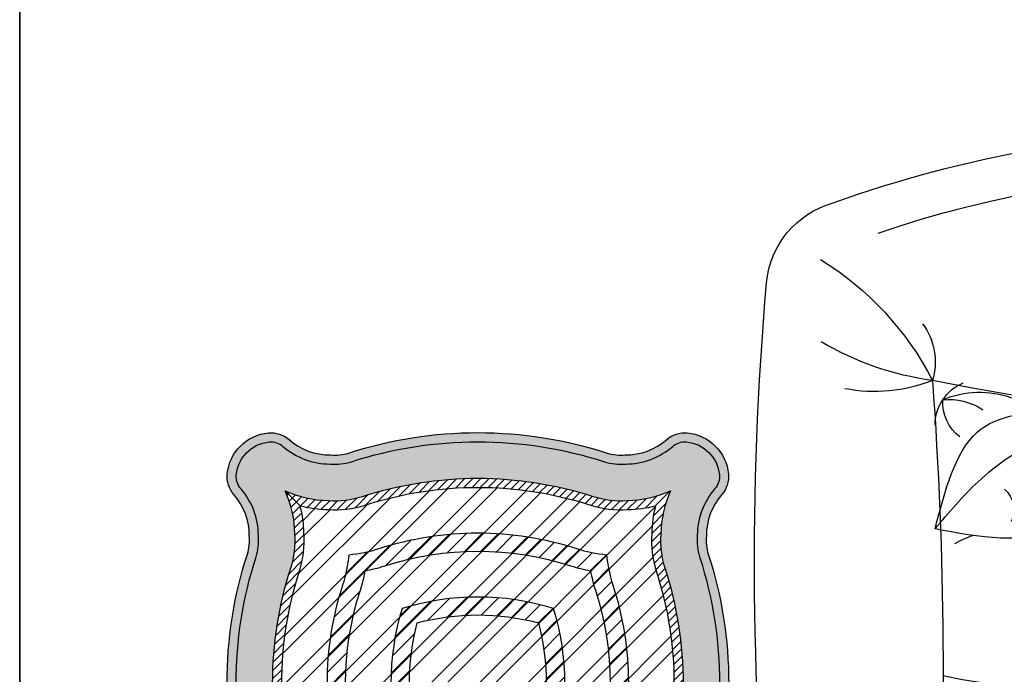
# Model space of a CAD drawing. Units: inches. Extents: x 844 to 2234, y 346 to 1084.
# Tile 63 of 93: x 1843.1 to 1860.31, y 724.36 to 735.81. Entities that reach past the tile are written whole.
import ezdxf

# ---------------------------------------------------------------- set-up
doc = ezdxf.new("R2010")
doc.units = ezdxf.units.IN
doc.header["$MEASUREMENT"] = 0
doc.layers.add('A-WALL', color=7, linetype='Continuous', lineweight=35)
doc.layers.add('furniture', color=8, linetype='Continuous', lineweight=18)
for name, color, linetype in [('RA-AP-01$0$FURN', 3, 'Continuous'), ('RA-AP-01$0$steel', 193, 'Continuous'), ('RA-AP-01$0$WOOD', 64, 'Continuous')]:
    doc.layers.add(name, color=color, linetype=linetype)
pattern_1 = [(45, (0, 1.362436106329781), (-0.0088388347648318, 0.0088388347648318), [])]
pattern_2 = [(45, (0, 1.362436106329781), (-0.0044194173824159, 0.0044194173824159), [])]

# ---------------------------------------------------------------- blocks, each defined once
blk = doc.blocks.new('A$C2FCF5309')
at = {"layer": 'RA-AP-01$0$FURN'}
h = blk.add_hatch(dxfattribs=at)
h.set_pattern_fill('ANSI31', color=256, scale=0.1, style=0)
h.set_pattern_definition(pattern_1)
h.paths.add_polyline_path([(5.038683893313746, -5.169250834004607, -0.1583983521602212), (5.038683893312098, -5.373464580902012, 0.0306258898943267), (5.033304057242972, -5.394827569605182, 0.0306258898948892), (5.01194106853941, -5.40020740567441, -0.1028142994996694), (4.878286182323899, -5.414871334512708), (4.863600873530158, -5.43331743520547, 0.1120482678681049), (5.018059823131753, -5.419248541734471, -0.052642197802937), (5.050972078299936, -5.412495590662115, -0.0526421977994963), (5.057725029371615, -5.379583335496025, 0.1583028414702701), (5.057725029372958, -5.163132079409654, -0.052642197806903), (5.050972078299777, -5.130219824239078, -0.0526421977995126), (5.018059823133679, -5.123466873167369, 0.0215995840215353), (4.988903013548211, -5.115372132362452), (4.975007495303644, -5.132826183367946, -0.0289147572844802), (5.011941068537408, -5.142508009226167, 0.0306258898976746), (5.033304057242868, -5.147887845296027, 0.0306258899022411)])
h.paths.add_polyline_path([(4.975007495303645, -5.132826183367946), (4.988903013548211, -5.115372132362452, 0.1362374241599938), (4.801608567045604, -5.12346687316654, -0.0526421978036853), (4.768696311876971, -5.130219824239102, -0.05264219780204), (4.761943360804856, -5.163132079406747, 0.1583028414743723), (4.761943360806116, -5.379583335498449, -0.0526421977955461), (4.768696311877141, -5.412495590662114, -0.0526421978073986), (4.801608567048022, -5.419248541735437, 0.0454484293938888), (4.863600873530158, -5.43331743520547), (4.878286182323899, -5.414871334512708, -0.0546933379798044), (4.80772732164382, -5.40020740567649, 0.030625889903973), (4.786364332934043, -5.394827569605216, 0.0306258898932853), (4.780984496865101, -5.373464580902791, -0.1583983521638281), (4.780984496864308, -5.169250834000963, 0.03062588989692), (4.786364332933943, -5.147887845296004, 0.0306258898946324), (4.807727321637318, -5.142508009226805, -0.1288932573266927)])
h.paths.add_polyline_path([(4.843422214712861, -5.204945727074827, -0.0783685831716868), (4.924134454130224, -5.196727409635105), (4.939146578618322, -5.177870798323143, 0.1012675676854134), (4.827248748758957, -5.188772261120899, 0.1253648873081696), (4.820394258584192, -5.327034652050361), (4.837127701354095, -5.306015906404253, -0.0981593964869636)], flags=17)
h.paths.add_polyline_path([(4.843422214712824, -5.337769687826355, -0.0311091841722656), (4.837127701354095, -5.306015906404253), (4.820394258584193, -5.32703465205036, 0.0247727657431944), (4.827248748758908, -5.353943153780261, 0.0812754385032542), (4.916962478476905, -5.36629034358622), (4.933684093813825, -5.345286454285511, -0.0876255421014372)], flags=17)
h.paths.add_polyline_path([(4.992419641418037, -5.353943153780226, 0.1506053783834298), (4.992419641417933, -5.188772261120954, 0.0485966419124224), (4.939146578618321, -5.177870798323143), (4.924134454130224, -5.196727409635105, -0.0507799419579301), (4.976246175464031, -5.204945727074882, -0.1296645318906876), (4.97624617546411, -5.337769687826316, -0.0415667119298777), (4.933684093813825, -5.345286454285511), (4.916962478476905, -5.36629034358622, 0.0684915676023693)], flags=17)
h = blk.add_hatch(dxfattribs=at)
h.set_pattern_fill('ANSI31', color=256, scale=0.1, style=0)
h.set_pattern_definition(pattern_1)
h.paths.add_polyline_path([(5.038683893313746, -5.169250834004607, -0.1583983521602212), (5.038683893312098, -5.373464580902012, 0.0306258898943267), (5.033304057242972, -5.394827569605182, 0.0306258898948892), (5.01194106853941, -5.40020740567441, -0.1028142994996694), (4.878286182323899, -5.414871334512708), (4.863600873530158, -5.43331743520547, 0.1120482678681049), (5.018059823131753, -5.419248541734471, -0.052642197802937), (5.050972078299936, -5.412495590662115, -0.0526421977994963), (5.057725029371615, -5.379583335496025, 0.1583028414702701), (5.057725029372958, -5.163132079409654, -0.052642197806903), (5.050972078299777, -5.130219824239078, -0.0526421977995126), (5.018059823133679, -5.123466873167369, 0.0215995840215353), (4.988903013548211, -5.115372132362452), (4.975007495303644, -5.132826183367946, -0.0289147572844802), (5.011941068537408, -5.142508009226167, 0.0306258898976746), (5.033304057242868, -5.147887845296027, 0.0306258899022411)])
h.paths.add_polyline_path([(4.975007495303645, -5.132826183367946), (4.988903013548211, -5.115372132362452, 0.1362374241599938), (4.801608567045604, -5.12346687316654, -0.0526421978036853), (4.768696311876971, -5.130219824239102, -0.05264219780204), (4.761943360804856, -5.163132079406747, 0.1583028414743723), (4.761943360806116, -5.379583335498449, -0.0526421977955461), (4.768696311877141, -5.412495590662114, -0.0526421978073986), (4.801608567048022, -5.419248541735437, 0.0454484293938888), (4.863600873530158, -5.43331743520547), (4.878286182323899, -5.414871334512708, -0.0546933379798044), (4.80772732164382, -5.40020740567649, 0.030625889903973), (4.786364332934043, -5.394827569605216, 0.0306258898932853), (4.780984496865101, -5.373464580902791, -0.1583983521638281), (4.780984496864308, -5.169250834000963, 0.03062588989692), (4.786364332933943, -5.147887845296004, 0.0306258898946324), (4.807727321637318, -5.142508009226805, -0.1288932573266927)])
h.paths.add_polyline_path([(4.843422214712861, -5.204945727074827, -0.0783685831716868), (4.924134454130224, -5.196727409635105), (4.939146578618322, -5.177870798323143, 0.1012675676854134), (4.827248748758957, -5.188772261120899, 0.1253648873081696), (4.820394258584192, -5.327034652050361), (4.837127701354095, -5.306015906404253, -0.0981593964869636)], flags=17)
h.paths.add_polyline_path([(4.843422214712824, -5.337769687826355, -0.0311091841722656), (4.837127701354095, -5.306015906404253), (4.820394258584193, -5.32703465205036, 0.0247727657431944), (4.827248748758908, -5.353943153780261, 0.0812754385032542), (4.916962478476905, -5.36629034358622), (4.933684093813825, -5.345286454285511, -0.0876255421014372)], flags=17)
h.paths.add_polyline_path([(4.992419641418037, -5.353943153780226, 0.1506053783834298), (4.992419641417933, -5.188772261120954, 0.0485966419124224), (4.939146578618321, -5.177870798323143), (4.924134454130224, -5.196727409635105, -0.0507799419579301), (4.976246175464031, -5.204945727074882, -0.1296645318906876), (4.97624617546411, -5.337769687826316, -0.0415667119298777), (4.933684093813825, -5.345286454285511), (4.916962478476905, -5.36629034358622, 0.0684915676023693)], flags=17)
at = {"layer": 'RA-AP-01$0$WOOD'}
h = blk.add_hatch(color=256, dxfattribs=at)
edge = h.paths.add_edge_path()
edge.add_arc((4.683001772622394, -5.026441828662609), 0.0299999999999998, 48.77105092035535, 95.25687599427813)
edge.add_arc((4.684834195088484, -5.046357707450686), 0.0499999999998897, 95.25687599443106, 174.7431240064049)
edge.add_arc((4.664918316300367, -5.044525284985046), 0.0300000000000005, 174.7431240062535, 221.2289490796905)
edge.add_arc((4.591236830209155, -5.109094338216345), 0.0679700159630267, -0.5333070513215148, 41.228949079691915, ccw=False)
edge.add_arc((4.609451302807284, -5.114694777173187), 0.0500000000000008, -17.3556839752095, 5.7020707654044145, ccw=False)
edge.add_arc((5.095208119646659, -5.271357707450659), 0.4603971832811796, 162.0683908477609, 197.9316091523306)
edge.add_arc((4.609451302807533, -5.428020637728902), 0.0500000000000006, -5.702070765320514, 17.355683975293914, ccw=False)
edge.add_arc((4.591236830209412, -5.433621076685779), 0.0679700159630261, -41.228949079600625, 0.5333070514128053, ccw=False)
edge.add_arc((4.664918316300727, -5.498190129916959), 0.0299999999999995, 138.7710509204022, 185.256875994324)
edge.add_arc((4.684834195088642, -5.496357707450695), 0.0499999999997451, 185.2568759946742, 264.74312400432)
edge.add_arc((4.683001772622394, -5.516273586238612), 0.03, 264.743124003969, 311.2289490796446)
edge.add_arc((4.747570825853633, -5.589955072329876), 0.0679700159630271, 89.4666929486321, 131.2289490796457, ccw=False)
edge.add_arc((4.753171264810493, -5.57174059973175), 0.0500000000000015, 72.64431602474701, 95.70207076536133, ccw=False)
edge.add_arc((4.909834195088355, -5.085983782892503), 0.4603971832811774, 252.0683908477147, 287.9316091522845)
edge.add_arc((5.06649712536621, -5.57174059973175), 0.0499999999999999, 84.29792923463953, 107.35568397525361, ccw=False)
edge.add_arc((5.072097564323069, -5.589955072329877), 0.0679700159630274, 48.771050920354185, 90.5333070513679, ccw=False)
edge.add_arc((5.136666617554309, -5.516273586238614), 0.0299999999999997, 228.771050920353, 275.2568759942969)
edge.add_arc((5.134834195088338, -5.496357707450417), 0.0499999999999982, 275.2568759942949, 354.7431240057633)
edge.add_arc((5.154750073876535, -5.498190129916372), 0.0299999999999999, 354.7431240057662, 401.2289490796891)
edge.add_arc((5.228431559967749, -5.433621076685074), 0.0679700159630274, 179.4666929486771, 221.2289490796903, ccw=False)
edge.add_arc((5.210217087369615, -5.428020637728227), 0.0499999999999976, 162.6443160247947, 185.7020707654089, ccw=False)
edge.add_arc((4.724460270530244, -5.271357707450757), 0.4603971832811793, 342.0683908477607, 377.9316091523305)
edge.add_arc((5.210217087369368, -5.114694777172509), 0.0500000000000019, 174.2979292346878, 197.355683975302, ccw=False)
edge.add_arc((5.228431559967489, -5.109094338215639), 0.0679700159630279, 138.7710509203993, 180.5333070514128, ccw=False)
edge.add_arc((5.154750073876174, -5.044525284984457), 0.0300000000000001, 318.771050920401, 365.2568759954636)
edge.add_arc((5.13483419508816, -5.046357707450624), 0.0499999999998349, 5.256875995237118, 84.74312400549572)
edge.add_arc((5.136666617554308, -5.026441828662608), 0.0299999999999994, 84.74312400572185, 131.2289490796446)
edge.add_arc((5.072097564323072, -4.952760342571343), 0.0679700159630261, 269.4666929486298, 311.22894907964354, ccw=False)
edge.add_arc((5.066497125366206, -4.97097481516947), 0.0499999999999992, 252.64431602475162, 275.70207076536565, ccw=False)
edge.add_arc((4.909834195088355, -5.456731632008717), 0.4603971832811764, 72.06839084771546, 107.9316091522853)
edge.add_arc((4.753171264810493, -4.970974815169471), 0.0500000000000016, 264.2979292346387, 287.355683975253, ccw=False)
edge.add_arc((4.747570825853633, -4.952760342571346), 0.0679700159630274, 228.7710509203543, 270.5333070513679, ccw=False)
edge = h.paths.add_edge_path(flags=16)
edge.add_arc((4.683001772622395, -5.026441828662608), 0.019999999999999, 48.7710509203555, 95.2568759942793)
edge.add_arc((4.684834195088469, -5.046357707450671), 0.0399999999998731, 95.2568759944489, 174.7431240064248)
edge.add_arc((4.664918316300404, -5.044525284985035), 0.020000000000036, 174.7431240062186, 221.2289490796461)
edge.add_arc((4.591236830209151, -5.109094338216346), 0.0779700159630296, -0.13764630038667747, 41.228949079689585, ccw=False)
edge.add_arc((4.609451302807307, -5.11469477717304), 0.060000000000024, -17.406127045137907, 5.176192161068002, ccw=False)
edge.add_arc((5.09520811964665, -5.271357707450659), 0.4503971832811708, 162.0623235129628, 197.9376764869162)
edge.add_arc((4.609451302807532, -5.428020637728943), 0.0599999999999982, -5.176192160466428, 17.406127046715312, ccw=False)
edge.add_arc((4.591236830209414, -5.433621076685778), 0.0779700159630257, -41.2289490796029, 0.13764630095249686, ccw=False)
edge.add_arc((4.664918316300731, -5.498190129916961), 0.0200000000000047, 138.7710509204103, 185.2568759943212)
edge.add_arc((4.684834195088606, -5.496357707450731), 0.0399999999997066, 185.2568759947174, 264.7431240043665)
edge.add_arc((4.683001772622369, -5.516273586238541), 0.020000000000069, 264.7431240038842, 311.2289490795622)
edge.add_arc((4.747570825853635, -5.589955072329884), 0.0779700159630344, 89.8623536987642, 131.2289490796432, ccw=False)
edge.add_arc((4.753171264810603, -5.571740599731771), 0.0599999999999895, 72.5938729544394, 95.1761921602253, ccw=False)
edge.add_arc((4.909834195088365, -5.085983782892505), 0.4503971832811724, 252.0623235129989, 287.9376764870498)
edge.add_arc((5.066497125366216, -5.571740599731755), 0.0600000000000047, 84.8238078399923, 107.40612704528041, ccw=False)
edge.add_arc((5.072097564322998, -5.589955072329853), 0.077970015963056, 48.771050920303594, 90.13764630126451, ccw=False)
edge.add_arc((5.136666617554307, -5.516273586238622), 0.0199999999999931, 228.771050920344, 275.2568759943037)
edge.add_arc((5.134834195088338, -5.496357707450416), 0.0400000000000004, 275.2568759942928, 354.7431240057607)
edge.add_arc((5.154750073876533, -5.498190129916375), 0.0200000000000037, 354.7431240057783, 401.2289490796939)
edge.add_arc((5.228431559967745, -5.433621076685076), 0.0779700159630239, 179.8623536995147, 221.2289490796908, ccw=False)
edge.add_arc((5.210217087369586, -5.428020637728345), 0.0600000000000054, 162.5938729554486, 185.1761921609759, ccw=False)
edge.add_arc((4.724460270530243, -5.271357707450766), 0.4503971832811826, 342.0623235128896, 377.937676486982)
edge.add_arc((5.210217087369347, -5.114694777172486), 0.0599999999999777, 174.8238078387611, 197.4061270462219, ccw=False)
edge.add_arc((5.228431559967523, -5.109094338215542), 0.0779700159629885, 138.7710509204687, 180.1376463004423, ccw=False)
edge.add_arc((5.154750073876175, -5.044525284984459), 0.0199999999999989, 318.771050920406, 365.2568759954698)
edge.add_arc((5.134834195088138, -5.046357707450646), 0.0399999999998586, 5.256875995208452, 84.74312400546732)
edge.add_arc((5.136666617554292, -5.02644182866256), 0.0199999999999529, 84.74312400577769, 131.2289490797025)
edge.add_arc((5.072097564323069, -4.952760342571338), 0.077970015963032, 269.86235369901414, 311.2289490796421, ccw=False)
edge.add_arc((5.06649712536618, -4.97097481516946), 0.0600000000000007, 252.5938729548277, 275.17619216047467, ccw=False)
edge.add_arc((4.909834195088353, -5.456731632008716), 0.4503971832811739, 72.06232351293887, 107.9376764867365)
edge.add_arc((4.753171264810429, -4.970974815169467), 0.0599999999999991, 264.82380783985815, 287.40612704769893, ccw=False)
edge.add_arc((4.747570825853681, -4.952760342571361), 0.0779700159630467, 228.7710509203206, 270.13764630113724, ccw=False)
h = blk.add_hatch(color=256, dxfattribs=at)
edge = h.paths.add_edge_path()
edge.add_arc((4.683001772622395, -5.026441828662608), 0.019999999999999, 48.7710509203555, 95.2568759942793)
edge.add_arc((4.684834195088469, -5.046357707450671), 0.0399999999998731, 95.2568759944489, 174.7431240064248)
edge.add_arc((4.664918316300404, -5.044525284985035), 0.020000000000036, 174.7431240062186, 221.2289490796461)
edge.add_arc((4.591236830209151, -5.109094338216346), 0.0779700159630296, -0.13764630038667747, 41.228949079689585, ccw=False)
edge.add_arc((4.609451302807307, -5.11469477717304), 0.060000000000024, -17.406127045137907, 5.176192161068002, ccw=False)
edge.add_arc((5.09520811964665, -5.271357707450659), 0.4503971832811708, 162.0623235129628, 197.9376764869162)
edge.add_arc((4.609451302807532, -5.428020637728943), 0.0599999999999982, -5.176192160466428, 17.406127046715312, ccw=False)
edge.add_arc((4.591236830209414, -5.433621076685778), 0.0779700159630257, -41.2289490796029, 0.13764630095249686, ccw=False)
edge.add_arc((4.664918316300731, -5.498190129916961), 0.0200000000000047, 138.7710509204103, 185.2568759943212)
edge.add_arc((4.684834195088606, -5.496357707450731), 0.0399999999997066, 185.2568759947174, 264.7431240043665)
edge.add_arc((4.683001772622369, -5.516273586238541), 0.020000000000069, 264.7431240038842, 311.2289490795622)
edge.add_arc((4.747570825853635, -5.589955072329884), 0.0779700159630344, 89.8623536987642, 131.2289490796432, ccw=False)
edge.add_arc((4.753171264810603, -5.571740599731771), 0.0599999999999895, 72.5938729544394, 95.1761921602253, ccw=False)
edge.add_arc((4.909834195088365, -5.085983782892505), 0.4503971832811724, 252.0623235129989, 287.9376764870498)
edge.add_arc((5.066497125366216, -5.571740599731755), 0.0600000000000047, 84.8238078399923, 107.40612704528041, ccw=False)
edge.add_arc((5.072097564322998, -5.589955072329853), 0.077970015963056, 48.771050920303594, 90.13764630126451, ccw=False)
edge.add_arc((5.136666617554307, -5.516273586238622), 0.0199999999999931, 228.771050920344, 275.2568759943037)
edge.add_arc((5.134834195088338, -5.496357707450416), 0.0400000000000004, 275.2568759942928, 354.7431240057607)
edge.add_arc((5.154750073876533, -5.498190129916375), 0.0200000000000037, 354.7431240057783, 401.2289490796939)
edge.add_arc((5.228431559967745, -5.433621076685076), 0.0779700159630239, 179.8623536995147, 221.2289490796908, ccw=False)
edge.add_arc((5.210217087369586, -5.428020637728345), 0.0600000000000054, 162.5938729554486, 185.1761921609759, ccw=False)
edge.add_arc((4.724460270530243, -5.271357707450766), 0.4503971832811826, 342.0623235128896, 377.937676486982)
edge.add_arc((5.210217087369347, -5.114694777172486), 0.0599999999999777, 174.8238078387611, 197.4061270462219, ccw=False)
edge.add_arc((5.228431559967523, -5.109094338215542), 0.0779700159629885, 138.7710509204687, 180.1376463004423, ccw=False)
edge.add_arc((5.154750073876175, -5.044525284984459), 0.0199999999999989, 318.771050920406, 365.2568759954698)
edge.add_arc((5.134834195088138, -5.046357707450646), 0.0399999999998586, 5.256875995208452, 84.74312400546732)
edge.add_arc((5.136666617554292, -5.02644182866256), 0.0199999999999529, 84.74312400577769, 131.2289490797025)
edge.add_arc((5.072097564323069, -4.952760342571338), 0.077970015963032, 269.86235369901414, 311.2289490796421, ccw=False)
edge.add_arc((5.06649712536618, -4.97097481516946), 0.0600000000000007, 252.5938729548277, 275.17619216047467, ccw=False)
edge.add_arc((4.909834195088353, -5.456731632008716), 0.4503971832811739, 72.06232351293887, 107.9376764867365)
edge.add_arc((4.753171264810429, -4.970974815169467), 0.0599999999999991, 264.82380783985815, 287.40612704769893, ccw=False)
edge.add_arc((4.747570825853681, -4.952760342571361), 0.0779700159630467, 228.7710509203206, 270.13764630113724, ccw=False)
edge = h.paths.add_edge_path(flags=16)
edge.add_arc((4.591236830209151, -5.109094338216348), 0.1179700159630308, 0.7417751874182841, 24.563326950263672, ccw=False)
edge.add_arc((4.609451302807302, -5.114694777173093), 0.100000000000012, -17.52836504564658, 4.087328884225087, ccw=False)
edge.add_arc((5.095208119646651, -5.271357707450657), 0.4103971832811724, 162.0403002448777, 197.9596997550675)
edge.add_arc((4.60945130280753, -5.428020637728918), 0.1000000000000027, -4.087328883827581, 17.528365046291924, ccw=False)
edge.add_arc((4.591236830209414, -5.433621076685779), 0.1179700159630246, 335.43667305041845, 359.2582248129738, ccw=False)
edge.add_arc((4.747570825853596, -5.589955072329891), 0.117970015963042, 90.7417751868461, 114.5633269496104, ccw=False)
edge.add_arc((4.753171264810559, -5.571740599731767), 0.0999999999999976, 72.47163495370341, 94.0873288836737, ccw=False)
edge.add_arc((4.909834195088367, -5.085983782892503), 0.4103971832811735, 252.0403002449999, 287.9596997551833)
edge.add_arc((5.066497125366205, -5.571740599731755), 0.1000000000000057, 85.91267111645209, 107.5283650455624, ccw=False)
edge.add_arc((5.072097564322985, -5.58995507232986), 0.117970015963046, 65.4366730497672, 89.25822481317113, ccw=False)
edge.add_arc((5.22843155996773, -5.433621076684992), 0.1179700159630096, 180.7417751873964, 204.5633269502712, ccw=False)
edge.add_arc((5.210217087369591, -5.428020637728301), 0.0999999999999969, 162.4716349546276, 184.0873288841682, ccw=False)
edge.add_arc((4.724460270530243, -5.271357707450766), 0.4103971832811825, 342.0403002448147, 377.9596997550345)
edge.add_arc((5.210217087369347, -5.114694777172489), 0.0999999999999796, 175.9126711156995, 197.5283650464392, ccw=False)
edge.add_arc((5.228431559967512, -5.109094338215525), 0.1179700159630019, 155.4366730502992, 179.2582248126247, ccw=False)
edge.add_arc((5.072097564323172, -4.952760342571314), 0.1179700159630537, 270.74177518697286, 294.56332694975765, ccw=False)
edge.add_arc((5.066497125366189, -4.970974815169462), 0.1000000000000017, 252.471634954247, 274.0873288838353, ccw=False)
edge.add_arc((4.909834195088353, -5.456731632008716), 0.4103971832811758, 72.04030024486342, 107.9596997549354)
edge.add_arc((4.75317126481046, -4.970974815169467), 0.1000000000000041, 265.91267111635307, 287.5283650466103, ccw=False)
edge.add_arc((4.747570825853629, -4.952760342571342), 0.1179700159630538, 245.43667304992562, 269.2582248131125, ccw=False)
h = blk.add_hatch(dxfattribs=at)
h.set_pattern_fill('ANSI31', color=256, scale=0.05, style=0)
h.set_pattern_definition(pattern_2)
h.paths.add_polyline_path([(5.105336294329346, -5.394854099602528, 0.0940138826956367), (5.100476366643778, -5.435568764288975, 0.0606271852326483), (5.104678567100611, -5.466202079462671, 0.0606271852344644), (5.074045251925975, -5.46199987900586, 0.0940138827021426), (5.033330587236848, -5.466859806692645, -0.1305325492494615), (4.828072633169377, -5.477944178050054), (4.821119726105699, -5.486677669841435, 0.1336226599878005), (5.036379334063467, -5.476383803188216, -0.0945969211935747), (5.073624810952389, -5.471994942692536, -0.1043170707892296), (5.121137550891356, -5.48266106325342, -0.1043170707868944), (5.110471430330457, -5.435148323315565, -0.0945969211952573), (5.114860290825935, -5.397902846425963, 0.1580239521433527), (5.114860290826324, -5.144812568476775, -0.0945969212010491), (5.110471430330247, -5.10756709158498, -0.1043170707844371), (5.121137550890657, -5.060054351648168, -0.104317070786514), (5.073624810952866, -5.070720472208642, -0.0945969211958523), (5.036379334063063, -5.066331611712874, 0.1580239521426795), (4.783289056114906, -5.066331611712465, -0.0945969211985319), (4.746043579224103, -5.070720472208672, -0.1043170707882665), (4.698530839285552, -5.060054351647925, -0.1043170707867205), (4.709196959846443, -5.10756709158571, -0.094596921196788), (4.704808099350826, -5.144812568475902, 0.1580239521433127), (4.704808099350699, -5.397902846425022, -0.094596921197841), (4.709196959846712, -5.435148323315576, -0.1043170707855109), (4.698530839286393, -5.482661063252921, -0.1043170707864168), (4.746043579224162, -5.471994942692571, -0.0945969211977586), (4.783289056114671, -5.476383803188671, 0.0238966994662183), (4.821119726105699, -5.486677669841435), (4.828072633169378, -5.477944178050054, -0.0269814195959459), (4.786337802940177, -5.466859806692736, 0.0940138827039629), (4.745623138250268, -5.461999879005895, 0.0606271852320776), (4.714989823076826, -5.466202079462476, 0.0606271852304618), (4.719192023533341, -5.435568764289856, 0.0940138826917763), (4.714332095848404, -5.394854099604977, -0.1580706864542086), (4.714332095846561, -5.147861315302034, 0.0940138827032017), (4.719192023533127, -5.107146650612438, 0.0606271852329446), (4.714989823076289, -5.076513335438588, 0.0606271852340035), (4.745623138250698, -5.08071553589536, 0.0940138827025969), (4.786337802940015, -5.075855608208526, -0.1580706864508517), (5.033330587237968, -5.075855608208939, 0.0940138827009578), (5.074045251926627, -5.080715535895319, 0.0606271852322557), (5.104678567100159, -5.076513335438697, 0.0606271852308743), (5.100476366643561, -5.107146650611519, 0.0940138827178109), (5.105336294331983, -5.147861315307182, -0.1580706864490946)])
h = blk.add_hatch(dxfattribs=at)
h.set_pattern_fill('ANSI31', color=256, scale=0.05, style=0)
h.set_pattern_definition(pattern_2)
h.paths.add_polyline_path([(5.105336294329346, -5.394854099602528, 0.0940138826956367), (5.100476366643778, -5.435568764288975, 0.0606271852326483), (5.104678567100611, -5.466202079462671, 0.0606271852344644), (5.074045251925975, -5.46199987900586, 0.0940138827021426), (5.033330587236848, -5.466859806692645, -0.1305325492494615), (4.828072633169377, -5.477944178050054), (4.821119726105699, -5.486677669841435, 0.1336226599878005), (5.036379334063467, -5.476383803188216, -0.0945969211935747), (5.073624810952389, -5.471994942692536, -0.1043170707892296), (5.121137550891356, -5.48266106325342, -0.1043170707868944), (5.110471430330457, -5.435148323315565, -0.0945969211952573), (5.114860290825935, -5.397902846425963, 0.1580239521433527), (5.114860290826324, -5.144812568476775, -0.0945969212010491), (5.110471430330247, -5.10756709158498, -0.1043170707844371), (5.121137550890657, -5.060054351648168, -0.104317070786514), (5.073624810952866, -5.070720472208642, -0.0945969211958523), (5.036379334063063, -5.066331611712874, 0.1580239521426795), (4.783289056114906, -5.066331611712465, -0.0945969211985319), (4.746043579224103, -5.070720472208672, -0.1043170707882665), (4.698530839285552, -5.060054351647925, -0.1043170707867205), (4.709196959846443, -5.10756709158571, -0.094596921196788), (4.704808099350826, -5.144812568475902, 0.1580239521433127), (4.704808099350699, -5.397902846425022, -0.094596921197841), (4.709196959846712, -5.435148323315576, -0.1043170707855109), (4.698530839286393, -5.482661063252921, -0.1043170707864168), (4.746043579224162, -5.471994942692571, -0.0945969211977586), (4.783289056114671, -5.476383803188671, 0.0238966994662183), (4.821119726105699, -5.486677669841435), (4.828072633169378, -5.477944178050054, -0.0269814195959459), (4.786337802940177, -5.466859806692736, 0.0940138827039629), (4.745623138250268, -5.461999879005895, 0.0606271852320776), (4.714989823076826, -5.466202079462476, 0.0606271852304618), (4.719192023533341, -5.435568764289856, 0.0940138826917763), (4.714332095848404, -5.394854099604977, -0.1580706864542086), (4.714332095846561, -5.147861315302034, 0.0940138827032017), (4.719192023533127, -5.107146650612438, 0.0606271852329446), (4.714989823076289, -5.076513335438588, 0.0606271852340035), (4.745623138250698, -5.08071553589536, 0.0940138827025969), (4.786337802940015, -5.075855608208526, -0.1580706864508517), (5.033330587237968, -5.075855608208939, 0.0940138827009578), (5.074045251926627, -5.080715535895319, 0.0606271852322557), (5.104678567100159, -5.076513335438697, 0.0606271852308743), (5.100476366643561, -5.107146650611519, 0.0940138827178109), (5.105336294331983, -5.147861315307182, -0.1580706864490946)])
h = blk.add_hatch(dxfattribs=at)
h.set_pattern_fill('ANSI32,_I', color=256, scale=0.1, style=2)
h.set_pattern_definition([(45, (0, 0), (-0.0265165042944955, 0.0265165042944955), []), (45, (0.0176776695, 0), (-0.0265165042944955, 0.0265165042944955), [])])
h.paths.add_polyline_path([(4.843422214712824, -5.337769687826354, 0.1296645318905289), (4.97624617546411, -5.337769687826316, 0.1296645318906876), (4.976246175464032, -5.204945727074882, 0.129664531890418), (4.843422214712861, -5.204945727074827, 0.129664531890765)], flags=0)
h.paths.add_polyline_path([(5.039131224122924, -5.170637849998464, -0.0326520429852175), (5.033304057242868, -5.147887845296027, -0.0326520429894721), (5.010554052537512, -5.142060678415043, 0.1561383235202698), (4.809114337641437, -5.142060678414318, -0.0326520429925972), (4.786364332933944, -5.147887845296004, -0.0326520429914489), (4.780537166052582, -5.170637850002729, 0.1561383235189577), (4.780537166052134, -5.37207756489719, -0.0326520429934175), (4.786364332934042, -5.394827569605215, -0.0326520429823496), (4.809114337634529, -5.400654736484653, 0.156138323524066), (5.010554052535268, -5.400654736486903, -0.032652042992888), (5.033304057242972, -5.394827569605183, -0.0326520429928733), (5.039131224124712, -5.372077564897496, 0.1561383235226786)], flags=0)
h.paths.add_polyline_path([(4.992419641418037, -5.353943153780226, -0.1506053783832862), (4.827248748758909, -5.353943153780261, -0.1506053783835069), (4.827248748758957, -5.188772261120899, -0.1506053783831346), (4.992419641417933, -5.188772261120954, -0.1506053783834298)], flags=0)
h.paths.add_polyline_path([(4.976246175464111, -5.337769687826316, -0.1296645318905298), (4.843422214712824, -5.337769687826354, -0.129664531890765), (4.843422214712862, -5.204945727074827, -0.1296645318904162), (4.976246175464031, -5.204945727074882, -0.1296645318906876)], flags=0)
h.paths.add_polyline_path([(5.105721254232479, -5.149054940982025, -0.0968902512052664), (5.100476366643561, -5.107146650611519, -0.0606271852308743), (5.104678567100159, -5.076513335438697, -0.0606271852322574), (5.074045251926626, -5.080715535895319, -0.0968902512197216), (5.032136961550132, -5.075470648304253, 0.1564657949319774), (4.787531428625239, -5.075470648304682, -0.0968902512150626), (4.745623138250699, -5.08071553589536, -0.060627185234009), (4.714989823076288, -5.076513335438587, -0.0606271852329501), (4.719192023533127, -5.10714665061244, -0.0968902512185585), (4.713947135942331, -5.149054940988458, 0.1564657949285579), (4.713947135940853, -5.393660473908259, -0.0968902512319826), (4.71919202353334, -5.435568764289873, -0.0606271852304288), (4.714989823076825, -5.466202079462476, -0.0606271852320811), (4.745623138250269, -5.461999879005895, -0.0968902512162649), (4.787531428625332, -5.467244766596559, 0.1564657949327057), (5.032136961551311, -5.46724476659659, -0.0968902512153659), (5.074045251925975, -5.46199987900586, -0.0606271852344627), (5.10467856710061, -5.466202079462671, -0.0606271852326483), (5.100476366643777, -5.435568764288975, -0.0968902512258216), (5.105721254235559, -5.393660473909953, 0.1564657949340142)])
h.paths.add_polyline_path([(5.057725029371625, -5.379583335495999, 0.0526421977995391), (5.050972078299936, -5.412495590662114, 0.0526421978029782), (5.018059823131728, -5.419248541734479, -0.1583028414681072), (4.801608567048168, -5.419248541735485, 0.0526421978076402), (4.76869631187714, -5.412495590662113, 0.0526421977956189), (4.761943360806101, -5.379583335498404, -0.1583028414743129), (4.761943360804846, -5.163132079406778, 0.0526421978020944), (4.768696311876972, -5.130219824239101, 0.0526421978033651), (4.80160856704541, -5.123466873166602, -0.1583028414716875), (5.018059823133628, -5.123466873167353, 0.0526421977995944), (5.050972078299776, -5.130219824239078, 0.0526421978070423), (5.057725029372986, -5.163132079409739, -0.1583028414701848)], flags=16)
h.paths.add_polyline_path([(5.038683893312112, -5.373464580901968, 0.0306258898943915), (5.033304057242972, -5.394827569605182, 0.0306258898948892), (5.01194106853941, -5.40020740567441, -0.1583983521587032), (4.807727321643864, -5.400207405676503, 0.0306258899040366), (4.786364332934043, -5.394827569605215, 0.0306258898931986), (4.780984496865119, -5.37346458090285, -0.1583983521638542), (4.7809844968643, -5.169250834000989, 0.0306258898969596), (4.786364332933945, -5.147887845296004, 0.0306258898946195), (4.807727321637311, -5.142508009226808, -0.1583983521623412), (5.011941068537318, -5.142508009226139, 0.030625889897807), (5.033304057242868, -5.147887845296028, 0.0306258899020632), (5.038683893313706, -5.169250834004486, -0.1583983521602835)], flags=0)
for p, q in [((4.714989823076289, -5.076513335438588), (4.698530839285552, -5.060054351647925)), ((4.714989823076289, -5.076513335438588), (4.698530839285552, -5.060054351647925)), ((5.104678567100159, -5.076513335438697), (5.121137550890656, -5.060054351648169)), ((5.104678567100159, -5.076513335438697), (5.121137550890656, -5.060054351648169)), ((5.10467856710061, -5.466202079462671), (5.121137550891355, -5.482661063253419)), ((5.10467856710061, -5.466202079462671), (5.121137550891355, -5.482661063253419))]:
    blk.add_line(p, q, dxfattribs=at)
for points in [[(4.702773858784635, -5.003879368495489, 0.2056608120285223), (4.680253138923443, -4.996568010480312, 0.3614336704708569), (4.635044498118043, -5.041776651286372, 0.2056608120263112), (4.642355856133262, -5.064297371147306, -0.1842662638101064), (4.65920390179375, -5.10972699154053, -0.1009492694051416), (4.657174869772992, -5.129609908955028, 0.1577727036674954), (4.657174869773219, -5.41310550594699, -0.1009492694051416), (4.659203901794006, -5.432988423361486, -0.1842662638101064), (4.64235585613359, -5.478418043754737, 0.2056608120285221), (4.635044498118431, -5.500938763615934, 0.3614336704593693), (4.680253138922529, -5.546147404420826, 0.2056608120364936), (4.702773858784635, -5.538836046405732, -0.1842662638101064), (4.748203479177874, -5.52198800074528, -0.1009492694051415), (4.768086396592371, -5.524017032766053, 0.1577727036674954), (5.051581993584332, -5.524017032766055, -0.1009492694051416), (5.071464910998829, -5.521988000745282, -0.1842662638101064), (5.116894531392067, -5.538836046405734, 0.2056608120286145), (5.13941525125327, -5.546147404420911, 0.3614336704683636), (5.184623892058835, -5.500938763615299, 0.2056608120285223), (5.177312534043641, -5.478418043754112, -0.1842662638101063), (5.160464488383153, -5.432988423360887, -0.1009492694051416), (5.162493520403909, -5.41310550594639, 0.1577727036674954), (5.162493520403684, -5.129609908954428, -0.1009492694051416), (5.160464488382894, -5.109726991539933, -0.1842662638101064), (5.17731253404331, -5.064297371146681, 0.2056608120337072), (5.184623892058415, -5.041776651284888, 0.3614336704623863), (5.139415251253259, -4.99656801048031, 0.2056608120285223), (5.116894531392067, -5.003879368495487, -0.1842662638101064), (5.071464910998829, -5.020727414155937, -0.1009492694051416), (5.051581993584332, -5.018698382135166, 0.1577727036674956), (4.768086396592371, -5.018698382135168, -0.1009492694051416), (4.748203479177874, -5.020727414155941, -0.1842662638101064)], [(4.702773858784635, -5.003879368495489, 0.2056608120285223), (4.680253138923443, -4.996568010480312, 0.3614336704708569), (4.635044498118043, -5.041776651286372, 0.2056608120263112), (4.642355856133262, -5.064297371147306, -0.1842662638101064), (4.65920390179375, -5.10972699154053, -0.1009492694051416), (4.657174869772992, -5.129609908955028, 0.1577727036674954), (4.657174869773219, -5.41310550594699, -0.1009492694051416), (4.659203901794006, -5.432988423361486, -0.1842662638101064), (4.64235585613359, -5.478418043754737, 0.2056608120285221), (4.635044498118431, -5.500938763615934, 0.3614336704593693), (4.680253138922529, -5.546147404420826, 0.2056608120364936), (4.702773858784635, -5.538836046405732, -0.1842662638101064), (4.748203479177874, -5.52198800074528, -0.1009492694051415), (4.768086396592371, -5.524017032766053, 0.1577727036674954), (5.051581993584332, -5.524017032766055, -0.1009492694051416), (5.071464910998829, -5.521988000745282, -0.1842662638101064), (5.116894531392067, -5.538836046405734, 0.2056608120286145), (5.13941525125327, -5.546147404420911, 0.3614336704683636), (5.184623892058835, -5.500938763615299, 0.2056608120285223), (5.177312534043641, -5.478418043754112, -0.1842662638101063), (5.160464488383153, -5.432988423360887, -0.1009492694051416), (5.162493520403909, -5.41310550594639, 0.1577727036674954), (5.162493520403684, -5.129609908954428, -0.1009492694051416), (5.160464488382894, -5.109726991539933, -0.1842662638101064), (5.17731253404331, -5.064297371146681, 0.2056608120337072), (5.184623892058415, -5.041776651284888, 0.3614336704623863), (5.139415251253259, -4.99656801048031, 0.2056608120285223), (5.116894531392067, -5.003879368495487, -0.1842662638101064), (5.071464910998829, -5.020727414155937, -0.1009492694051416), (5.051581993584332, -5.018698382135166, 0.1577727036674956), (4.768086396592371, -5.018698382135168, -0.1009492694051416), (4.748203479177874, -5.020727414155941, -0.1842662638101064)], [(4.696183163397222, -5.011400188551196, 0.2056608120285295), (4.681169350156427, -5.006525949874411, 0.3614336704708588), (4.645002437512154, -5.042692862519237, 0.2056608120262659), (4.649876676188964, -5.057706675759887, -0.182481815856965), (4.669206621172843, -5.109281651732388, -0.0988540857970112), (4.666703803477437, -5.13264334722805, 0.1578269695851905), (4.666703803477144, -5.410072067672365, -0.0988540858013112), (4.6692066211731, -5.433433763168966, -0.1824818158591246), (4.649876676189301, -5.485008739142145, 0.2056608120284717), (4.64500243751253, -5.500022552382944, 0.3614336704593821), (4.681169350155757, -5.536189465026749, 0.2056608120365057), (4.696183163397221, -5.531315226350026, -0.1824818158605826), (4.747758139370833, -5.51198528136619, -0.0988540857951607), (4.771119834866025, -5.514488099061806, 0.1578269695856264), (5.04854855531107, -5.514488099061688, -0.0988540857929677), (5.071910250805761, -5.511985281366138, -0.1824818158609529), (5.123485226779481, -5.531315226350027, 0.2056608120286893), (5.138499040020282, -5.536189465026812, 0.3614336704683556), (5.174665952664737, -5.500022552382323, 0.2056608120284882), (5.169791713987938, -5.485008739141532, -0.1824818158574124), (5.150461769004059, -5.4334337631689, -0.0988540857940221), (5.152964586699289, -5.410072067673927, 0.1578269695858123), (5.1529645866996, -5.132643347228565, -0.0988540858025403), (5.150461769003872, -5.109281651731659, -0.1824818158565006), (5.169791713987599, -5.057706675759273, 0.2056608120337192), (5.174665952664335, -5.042692862518078, 0.3614336704623903), (5.138499040020236, -5.006525949874406, 0.2056608120285323), (5.123485226779481, -5.011400188551195, -0.1824818158594503), (5.071910250806212, -5.03073013353503, -0.09885408579455), (5.048548555311143, -5.028227315839558, 0.1578269695844942), (4.771119834867991, -5.028227315838772, -0.0988540858042156), (4.747758139370745, -5.030730133535067, -0.1824818158603032)], [(4.696183163397222, -5.011400188551196, 0.2056608120285295), (4.681169350156427, -5.006525949874411, 0.3614336704708588), (4.645002437512154, -5.042692862519237, 0.2056608120262659), (4.649876676188964, -5.057706675759887, -0.182481815856965), (4.669206621172843, -5.109281651732388, -0.0988540857970112), (4.666703803477437, -5.13264334722805, 0.1578269695851905), (4.666703803477144, -5.410072067672365, -0.0988540858013112), (4.6692066211731, -5.433433763168966, -0.1824818158591246), (4.649876676189301, -5.485008739142145, 0.2056608120284717), (4.64500243751253, -5.500022552382944, 0.3614336704593821), (4.681169350155757, -5.536189465026749, 0.2056608120365057), (4.696183163397221, -5.531315226350026, -0.1824818158605826), (4.747758139370833, -5.51198528136619, -0.0988540857951607), (4.771119834866025, -5.514488099061806, 0.1578269695856264), (5.04854855531107, -5.514488099061688, -0.0988540857929677), (5.071910250805761, -5.511985281366138, -0.1824818158609529), (5.123485226779481, -5.531315226350027, 0.2056608120286893), (5.138499040020282, -5.536189465026812, 0.3614336704683556), (5.174665952664737, -5.500022552382323, 0.2056608120284882), (5.169791713987938, -5.485008739141532, -0.1824818158574124), (5.150461769004059, -5.4334337631689, -0.0988540857940221), (5.152964586699289, -5.410072067673927, 0.1578269695858123), (5.1529645866996, -5.132643347228565, -0.0988540858025403), (5.150461769003872, -5.109281651731659, -0.1824818158565006), (5.169791713987599, -5.057706675759273, 0.2056608120337192), (5.174665952664335, -5.042692862518078, 0.3614336704623903), (5.138499040020236, -5.006525949874406, 0.2056608120285323), (5.123485226779481, -5.011400188551195, -0.1824818158594503), (5.071910250806212, -5.03073013353503, -0.09885408579455), (5.048548555311143, -5.028227315839558, 0.1578269695844942), (4.771119834867991, -5.028227315838772, -0.0988540858042156), (4.747758139370745, -5.030730133535067, -0.1824818158603032)], [(4.698530839285552, -5.060054351647925, -0.1043170707867612), (4.709196959846444, -5.107567091585729, -0.0945969211969405), (4.704808099350802, -5.144812568475978, 0.1580239521432241), (4.704808099350681, -5.397902846424963, -0.0945969211980322), (4.709196959846711, -5.43514832331559, -0.104317070785482), (4.698530839286393, -5.482661063252921, -0.1043170707864036), (4.746043579224155, -5.471994942692571, -0.094596921197375), (4.78328905611452, -5.476383803188623, 0.1580239521431959), (5.036379334063463, -5.476383803188218, -0.0945969211935888), (5.07362481095239, -5.471994942692536, -0.1043170707892253), (5.121137550891355, -5.482661063253419, -0.1043170707868921), (5.110471430330457, -5.435148323315565, -0.0945969211954828), (5.114860290825962, -5.397902846425878, 0.158023952143358), (5.114860290826295, -5.144812568476682, -0.0945969212007617), (5.110471430330247, -5.107567091584995, -0.1043170707844689), (5.121137550890656, -5.060054351648169, -0.1043170707864946), (5.073624810952874, -5.070720472208642, -0.0945969211956941), (5.036379334063131, -5.066331611712896, 0.1580239521426976), (4.783289056114946, -5.066331611712452, -0.0945969211986379), (4.746043579224103, -5.070720472208672, -0.1043170707882684)], [(4.698530839285552, -5.060054351647925, -0.1043170707867612), (4.709196959846444, -5.107567091585729, -0.0945969211969405), (4.704808099350802, -5.144812568475978, 0.1580239521432241), (4.704808099350681, -5.397902846424963, -0.0945969211980322), (4.709196959846711, -5.43514832331559, -0.104317070785482), (4.698530839286393, -5.482661063252921, -0.1043170707864036), (4.746043579224155, -5.471994942692571, -0.094596921197375), (4.78328905611452, -5.476383803188623, 0.1580239521431959), (5.036379334063463, -5.476383803188218, -0.0945969211935888), (5.07362481095239, -5.471994942692536, -0.1043170707892253), (5.121137550891355, -5.482661063253419, -0.1043170707868921), (5.110471430330457, -5.435148323315565, -0.0945969211954828), (5.114860290825962, -5.397902846425878, 0.158023952143358), (5.114860290826295, -5.144812568476682, -0.0945969212007617), (5.110471430330247, -5.107567091584995, -0.1043170707844689), (5.121137550890656, -5.060054351648169, -0.1043170707864946), (5.073624810952874, -5.070720472208642, -0.0945969211956941), (5.036379334063131, -5.066331611712896, 0.1580239521426976), (4.783289056114946, -5.066331611712452, -0.0945969211986379), (4.746043579224103, -5.070720472208672, -0.1043170707882684)], [(4.714989823076289, -5.076513335438588, -0.0606271852329464), (4.719192023533127, -5.107146650612439, -0.0940138827030756), (4.714332095846578, -5.147861315301983, 0.1580706864542707), (4.714332095848417, -5.394854099605018, -0.0940138826916965), (4.719192023533341, -5.435568764289864, -0.0606271852304462), (4.714989823076826, -5.466202079462476, -0.0606271852320585), (4.745623138250258, -5.461999879005895, -0.0940138827037036), (4.786337802940059, -5.466859806692699, 0.1580706864500221), (5.033330587236783, -5.466859806692666, -0.0940138827023111), (5.074045251925979, -5.46199987900586, -0.060627185234454), (5.10467856710061, -5.466202079462671, -0.0606271852326709), (5.100476366643777, -5.435568764288963, -0.0940138826958686), (5.105336294329379, -5.394854099602421, 0.1580706864489859), (5.105336294331999, -5.147861315307237, -0.0940138827179432), (5.100476366643561, -5.107146650611518, -0.0606271852308726), (5.104678567100159, -5.076513335438697, -0.0606271852322592), (5.074045251926625, -5.080715535895319, -0.094013882701022), (5.03333058723794, -5.075855608208931, 0.1580706864508015), (4.786337802940061, -5.075855608208511, -0.0940138827027143), (4.745623138250695, -5.08071553589536, -0.0606271852339983)], [(4.714989823076289, -5.076513335438588, -0.0606271852329464), (4.719192023533127, -5.107146650612439, -0.0940138827030756), (4.714332095846578, -5.147861315301983, 0.1580706864542707), (4.714332095848417, -5.394854099605018, -0.0940138826916965), (4.719192023533341, -5.435568764289864, -0.0606271852304462), (4.714989823076826, -5.466202079462476, -0.0606271852320585), (4.745623138250258, -5.461999879005895, -0.0940138827037036), (4.786337802940059, -5.466859806692699, 0.1580706864500221), (5.033330587236783, -5.466859806692666, -0.0940138827023111), (5.074045251925979, -5.46199987900586, -0.060627185234454), (5.10467856710061, -5.466202079462671, -0.0606271852326709), (5.100476366643777, -5.435568764288963, -0.0940138826958686), (5.105336294329379, -5.394854099602421, 0.1580706864489859), (5.105336294331999, -5.147861315307237, -0.0940138827179432), (5.100476366643561, -5.107146650611518, -0.0606271852308726), (5.104678567100159, -5.076513335438697, -0.0606271852322592), (5.074045251926625, -5.080715535895319, -0.094013882701022), (5.03333058723794, -5.075855608208931, 0.1580706864508015), (4.786337802940061, -5.075855608208511, -0.0940138827027143), (4.745623138250695, -5.08071553589536, -0.0606271852339983)], [(4.768696311876972, -5.130219824239102, -0.0526421978019087), (4.761943360804882, -5.163132079406667, 0.1583028414744761), (4.761943360806133, -5.379583335498504, -0.0526421977954539), (4.76869631187714, -5.412495590662113, -0.0526421978076619), (4.801608567048181, -5.419248541735488, 0.1583028414681522), (5.0180598231318, -5.419248541734456, -0.0526421978028585), (5.050972078299936, -5.412495590662114, -0.0526421977992923), (5.057725029371576, -5.379583335496149, 0.1583028414703719), (5.057725029372956, -5.163132079409646, -0.0526421978068888), (5.050972078299776, -5.130219824239078, -0.052642197799403), (5.018059823133745, -5.12346687316739, 0.1583028414717216), (4.801608567045482, -5.123466873166579, -0.0526421978034837)], [(4.768696311876972, -5.130219824239102, -0.0526421978019087), (4.761943360804882, -5.163132079406667, 0.1583028414744761), (4.761943360806133, -5.379583335498504, -0.0526421977954539), (4.76869631187714, -5.412495590662113, -0.0526421978076619), (4.801608567048181, -5.419248541735488, 0.1583028414681522), (5.0180598231318, -5.419248541734456, -0.0526421978028585), (5.050972078299936, -5.412495590662114, -0.0526421977992923), (5.057725029371576, -5.379583335496149, 0.1583028414703719), (5.057725029372956, -5.163132079409646, -0.0526421978068888), (5.050972078299776, -5.130219824239078, -0.052642197799403), (5.018059823133745, -5.12346687316739, 0.1583028414717216), (4.801608567045482, -5.123466873166579, -0.0526421978034837)], [(4.786364332933944, -5.147887845296004, -0.0306258898969254), (4.780984496864308, -5.169250834000966, 0.1583983521638412), (4.780984496865107, -5.373464580902811, -0.0306258898932568), (4.786364332934043, -5.394827569605216, -0.0306258899041339), (4.80772732164393, -5.400207405676526, 0.1583983521586416), (5.011941068539401, -5.400207405674413, -0.0306258898949021), (5.033304057242972, -5.394827569605182, -0.0306258898943513), (5.038683893312104, -5.373464580901996, 0.1583983521602784), (5.038683893313717, -5.16925083400452, -0.0306258899021139), (5.033304057242868, -5.147887845296027, -0.030625889897777), (5.011941068537338, -5.142508009226145, 0.1583983521624288), (4.807727321637224, -5.142508009226835, -0.0306258898944937)], [(4.786364332933944, -5.147887845296004, -0.0306258898969254), (4.780984496864308, -5.169250834000966, 0.1583983521638412), (4.780984496865107, -5.373464580902811, -0.0306258898932568), (4.786364332934043, -5.394827569605216, -0.0306258899041339), (4.80772732164393, -5.400207405676526, 0.1583983521586416), (5.011941068539401, -5.400207405674413, -0.0306258898949021), (5.033304057242972, -5.394827569605182, -0.0306258898943513), (5.038683893312104, -5.373464580901996, 0.1583983521602784), (5.038683893313717, -5.16925083400452, -0.0306258899021139), (5.033304057242868, -5.147887845296027, -0.030625889897777), (5.011941068537338, -5.142508009226145, 0.1583983521624288), (4.807727321637224, -5.142508009226835, -0.0306258898944937)], [(4.827248748758957, -5.1887722611209, 0.1506053783835061), (4.827248748758908, -5.353943153780261, 0.150605378383287), (4.992419641418037, -5.353943153780226, 0.1506053783834298), (4.992419641417933, -5.188772261120954, 0.1506053783831346)], [(4.827248748758957, -5.1887722611209, 0.1506053783835061), (4.827248748758908, -5.353943153780261, 0.150605378383287), (4.992419641418037, -5.353943153780226, 0.1506053783834298), (4.992419641417933, -5.188772261120954, 0.1506053783831346)], [(4.843422214712861, -5.204945727074827, 0.1296645318907659), (4.843422214712824, -5.337769687826355, 0.1296645318905299), (4.976246175464111, -5.337769687826316, 0.1296645318906876), (4.976246175464032, -5.204945727074882, 0.129664531890418)], [(4.843422214712861, -5.204945727074827, 0.1296645318907659), (4.843422214712824, -5.337769687826355, 0.1296645318905299), (4.976246175464111, -5.337769687826316, 0.1296645318906876), (4.976246175464032, -5.204945727074882, 0.129664531890418)]]:
    blk.add_lwpolyline(points, format="xyb", close=True, dxfattribs=at)
blk = doc.blocks.new('A$C7F4351E2')
at = {"layer": 'RA-AP-01$0$FURN'}
for p, q in [((8.352559572600457, -8.263941955512525), (8.35255957259913, -8.282283310927069)), ((8.352559572600457, -8.927748273106442), (8.35255957259913, -8.909406917691898))]:
    blk.add_line(p, q, dxfattribs=at)
at = {"layer": 'RA-AP-01$0$FURN', "const_width": 0.01}
for points in [[(8.437812509519787, -8.415359762755768, 1), (8.427812509519786, -8.415359762755742, 1)], [(8.758197489244363, -8.415359762756214, -1), (8.768197489244365, -8.415359762756214, -1)], [(8.437812509519787, -8.776330465863198, -1), (8.427812509519786, -8.776330465863225, -1)], [(8.758197489244363, -8.776330465862753, 1), (8.768197489244365, -8.776330465862753, 1)]]:
    blk.add_lwpolyline(points, format="xyb", close=True, dxfattribs=at)
at = {"layer": 'RA-AP-01$0$FURN'}
for centre, radius, start, end in [((8.727559572604601, -11.61690445537682), 3.552808610866049, 85.0473312316413, 96.05887237565803), ((8.50205957259015, -8.17394195551301), 0.1744999999876311, 148.9517780040467, 211.048221995953), ((9.025650106946005, -8.176987401637472), 0.1, 15.499494600857, 85.04733123164159), ((8.77247054904813, -7.958543863781743), 0.3382138395168437, 297.2303327094027, 328.2563708342649), ((9.2484631175852, -8.302692737637487), 0.3241573581843151, 149.2985674842688, 172.3026350986055), ((7.88981694267423, -8.595845114309485), 1.310286319972027, 340.1192502251003, 19.8807497748998), ((9.084915705374858, -8.196040134964925), 0.1698955038956699, 168.877843135945, 201.8512383801196), ((7.929864357850293, -8.595845114309483), 1.224941341589781, 341.1257460634955, 18.87425393650447), ((8.947672844970796, -8.191835192646359), 0.0704710051510922, 253.1338634205325, 306.4126496157095), ((8.408522229993444, -8.33300072568355), 0.0753785023123622, 115.8745619060558, 163.9833547230034), ((8.603635103111959, -3.79706073025477), 4.473931917517753, 266.7828902523826, 274.1477233631118), ((8.878389979098333, -8.312202545234353), 0.05, 30.14777190425723, 89.99999999905349), ((10.52713941284929, -8.595845114309466), 1.634931324962266, 168.1200364254424, 191.8799635745573), ((9.101231010340802, -8.38034106221356), 0.5100538472773755, 167.6182489359307, 193.3122231353938), ((8.903279781571525, -8.31837865610295), 0.0478550828899777, 86.575295631534, 142.6833829238214), ((8.838100984994732, -8.276822957859652), 0.0683206773889159, 326.6729861493449, 5.218395042636973), ((8.810121490949696, -8.31110757721543), 0.1042084262671507, 340.4828318717155, 22.86929393278168), ((8.395364730619693, -8.304213854581548), 0.0479292786975047, 152.8070868543555, 225.4025460716553), ((8.333592787569726, -8.402663469525104), 0.1218651776285568, 48.0375529564433, 81.04623209541253), ((7.439612310514541, -8.913795367824825), 1.11020813118073, 31.93286085977143, 34.66647731879807), ((8.553131949433, -8.344109762755968), 0.1214118203512435, 150.1419074485596, 187.691663289156), ((8.642878049331348, -8.344109762756093), 0.1214118203512435, 352.3083367106845, 29.85809255128089), ((9.82633505008426, -8.696671375220811), 1.539060359583382, 165.5338783218257, 176.2437734318419), ((8.374918524725835, -8.294321202996931), 0.1212957045587361, 247.3375839744822, 273.7314750942433), ((8.546954810732721, -8.753394424755975), 0.3517162425384579, 83.41248966761125, 103.1674570565571), ((8.697701155637269, -8.172468128267624), 0.2442261434243043, 248.9017070735605, 275.9923925191661), ((8.73287643248165, -8.469775898206471), 0.3023568492824586, 173.0944825511667, 197.588060785551), ((8.889871101981017, -8.492307869305423), 0.1295083186917369, 167.9901339202812, 211.3796151021958), ((8.444145567704187, -7.829943385268752), 0.765467899454341, 258.6273206109321, 281.4174148186357), ((8.781211457338294, -7.772561243483908), 0.8232838708255751, 260.2449188973366, 277.7495311655964), ((9.82633505008426, -8.495018853398156), 1.539060359583382, 183.7562265681581, 194.4661216781742), ((8.444145567704187, -9.361312955433425), 0.765467899454341, 78.58258518136427, 101.3726793890678), ((8.781211457338294, -9.418695097218269), 0.8232838708255751, 82.25060502413102, 99.75508110266344), ((8.73287643248165, -8.721914330412496), 0.3023568492824586, 162.411939214449, 186.9055174488332), ((8.889871101981017, -8.699382359313544), 0.1295083186917369, 148.6203848978042, 192.0098660797188), ((9.101231010340802, -8.811349166405407), 0.5100538472773755, 166.6877768646062, 192.3817510640693), ((8.799643412436344, -8.749969313933361), 0.0689028341546707, 265.5384273543114, 353.5804828909086), ((8.374918524725835, -8.897369025622035), 0.1212957045587361, 86.26852490575668, 112.6624160255178), ((8.697701155637269, -9.019222100351342), 0.2442261434243043, 84.00760748083387, 111.0982929264395), ((8.546954810732721, -8.438295803862992), 0.3517162425384579, 256.8325429434429, 276.5875103323888), ((8.553131949433, -8.847580465862999), 0.1214118203512435, 172.308336710844, 209.8580925514404), ((8.785133372574222, -8.874256642962408), 0.0310151388417235, 42.62105484496073, 114.2239681486109), ((8.810121490949696, -8.880582651403534), 0.1042084262671507, 337.1307060672183, 19.51716812828453), ((8.395364730619693, -8.88747637403742), 0.0479292786975047, 134.5974539283447, 207.1929131456445), ((7.439612310514541, -8.277894860794142), 1.11020813118073, 325.333522681202, 328.0671391402286), ((8.408522229993444, -8.858689502935416), 0.0753785023123622, 196.0166452769965, 244.1254380939442), ((8.333592787569726, -8.789026759093863), 0.1218651776285568, 278.9537679045875, 311.9624470435567), ((8.838100984994732, -8.914867270759315), 0.0683206773889159, 354.781604957363, 33.32701385065517), ((8.642878049331348, -8.847580465862874), 0.1214118203512435, 330.1419074487191, 340.3913536181062), ((8.903279781571525, -8.873311572516016), 0.0478550828899777, 217.3166170761785, 273.424704368466), ((8.878389979098333, -8.879487683384612), 0.05, 270.0000000009465, 337.4173275753961), ((8.50205957259015, -9.017748273105955), 0.1744999999876311, 148.9517780040469, 211.0482219959533), ((8.603635103111959, -13.39462949836419), 4.473931917517753, 85.85227663688822, 93.21710974761734), ((9.084915705374858, -8.995650093654042), 0.1698955038956699, 158.1487616198804, 191.122156864055), ((8.947672844970796, -8.999855035972608), 0.0704710051510922, 53.58735038429053, 106.8661365794674), ((8.77247054904813, -9.233146364837223), 0.3382138395168437, 31.74362916573515, 62.76966729059727), ((9.2484631175852, -8.88899749098148), 0.3241573581843151, 187.6973649013944, 210.7014325157311), ((9.025650106946005, -9.014702826981493), 0.1, 274.9526687683584, 344.500505399143), ((8.727559572604601, -5.574785773242145), 3.552808610866049, 263.941127624342, 274.9526687683587)]:
    blk.add_arc(centre, radius, start, end, dxfattribs=at)
for points, knots in [([(8.764421239581775, -8.929562504990262), (8.755250524728652, -8.881106864374377), (8.74196437992213, -8.810906376383404), (8.80604948961138, -8.740469753734786), (8.847474678848357, -8.701097198289744), (8.897142214037096, -8.58322730303861), (8.897091569728207, -8.784804210134517), (8.88612504526093, -8.897825917224484), (8.806539053396843, -8.9185794820093), (8.764421239581775, -8.92956250499026)], [0, 0, 0, 0, 0.1367586589314792, 0.1981301758052368, 0.2677729570689282, 0.3281194902553322, 0.4737578340741565, 0.5765194025309516, 0.6920332287422236, 0.6920332287422236, 0.6920332287422236, 0.6920332287422236]), ([(8.764421239581775, -8.92956250499026), (8.782204778269502, -8.914603263160053), (8.821592007255505, -8.881471326160916), (8.86917941606436, -8.814322636989944), (8.867818990542759, -8.729338202119969), (8.881231406199264, -8.676770566934765), (8.888101821971249, -8.649843164808122)], [0, 0, 0, 0, 0.070018540671015, 0.1550780383534498, 0.2344491945777043, 0.3178048737568289, 0.3178048737568289, 0.3178048737568289, 0.3178048737568289])]:
    blk.add_open_spline(points, degree=3, knots=knots, dxfattribs=at)
blk = doc.blocks.new('A$C5D2F253E')
at = {"layer": 'RA-AP-01$0$steel', "xscale": -1}
blk.add_blockref('A$C2FCF5309', (6.339960502260055, 7.248884637679282), dxfattribs=at)
at = {"layer": 'RA-AP-01$0$WOOD', "xscale": -1, "rotation": 180}
blk.add_blockref('A$C7F4351E2', (-7.164808785335935, -7.45332973198748), dxfattribs=at)

msp = doc.modelspace()

# ---------------------------------------------------------------- linework, layer by layer
at = {"layer": 'A-WALL'}
msp.add_line((1843.099168352677, 766.4551697629895), (1843.099168352677, 629.4551697629895), dxfattribs=at)

# ---------------------------------------------------------------- block references
at = {"layer": 'furniture', "xscale": 15.94108302203742, "yscale": 15.94108302203742, "zscale": 15.94108302203742, "rotation": 90}
msp.add_blockref('A$C5D2F253E', (1882.631064852549, 701.4028671565849), dxfattribs=at)

doc.saveas('drawing.dxf')
